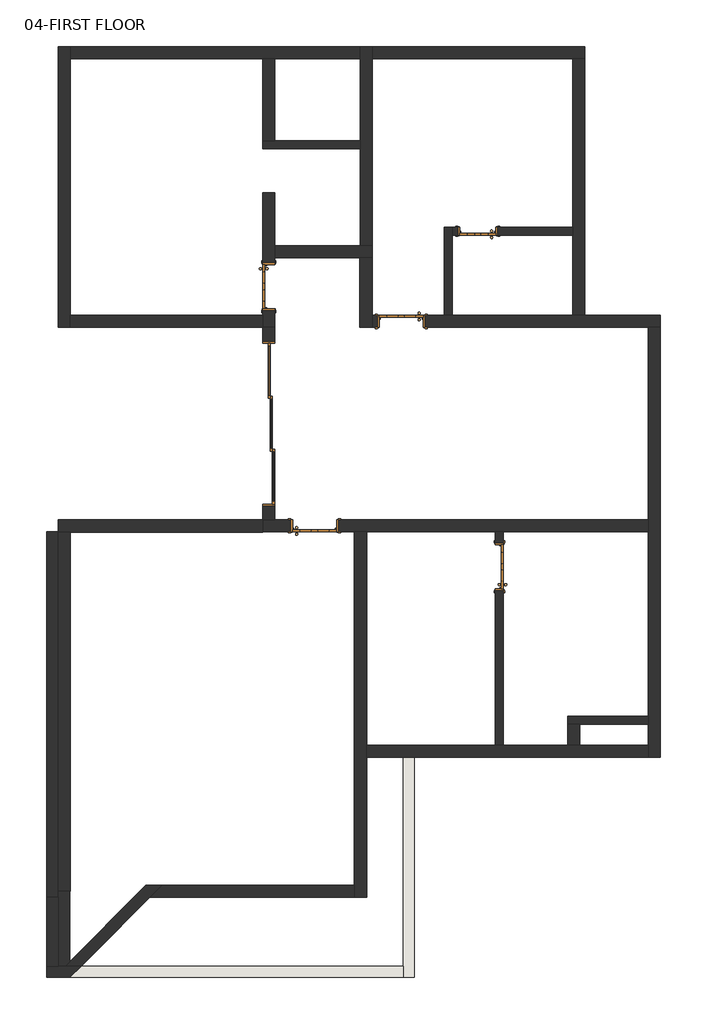
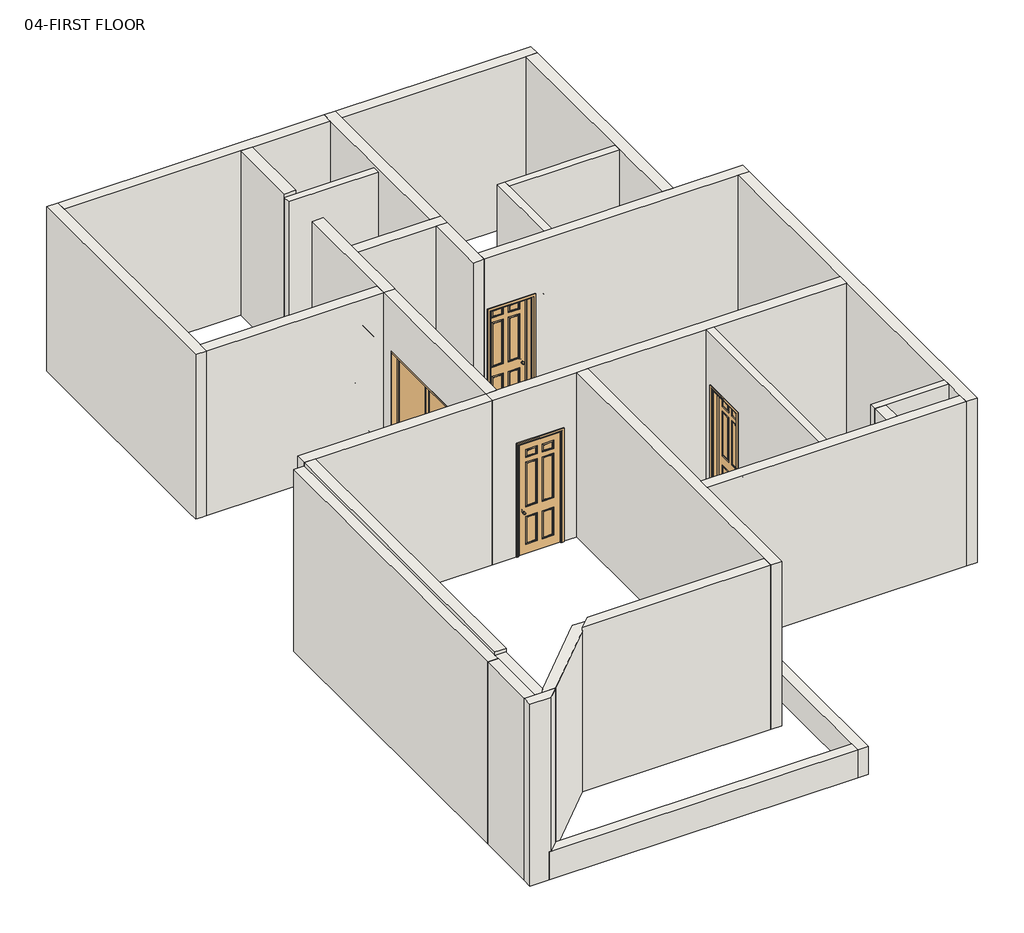
# One storey: 32 walls, 6 doors.
"""IFC4 building model written with IfcOpenShell, lengths in millimetres."""

from ifc_helpers import new_model, si_unit, frame, origin, place, context, project, spatial, polyline, outline, extrude, faceted_brep, transform, mapped, element, save
from components import d4_ba08b5a2, intsgl_9_d1_21fcec07, intsgl_9_d1_ea64c5f3, intsgl_9_d2_8283ee4d

model = new_model("IFC4")

# Units and contexts
model_context = context("Model", 3, world=origin())
ifc_project = project(units=[si_unit("LENGTHUNIT", "METRE", prefix="MILLI")], contexts=[model_context])

# Site, building, storey
site = spatial("IfcSite", under=ifc_project)
building = spatial("IfcBuilding", under=site)
storey = spatial("IfcBuildingStorey", under=building, Name="04-FIRST FLOOR", Elevation=4050.0)

# Doors
placement = place(None, origin())
d4_shape = d4_ba08b5a2(model_context)
element("IfcDoor", 1, ObjectType="D4", at=placement, inside=storey, context=model_context, shape_type="MappedRepresentation", body=[
    mapped(d4_shape, transform((-10636.6107921, -10590.6567046, 4050.0), x_axis=(0.0, 1.0, 0.0), y_axis=(-1.0, 0.0, 0.0), z_axis=(0.0, 0.0, 1.0))),
])
intsgl_9_d1_shape = intsgl_9_d1_21fcec07(model_context)
element("IfcDoor", 2, ObjectType="IntSgl (9) : D1", at=placement, inside=storey, context=model_context, shape_type="MappedRepresentation", body=[
    mapped(intsgl_9_d1_shape, transform((-8164.1107921, -8599.8987034, 4050.0), x_axis=(-1.0, 0.0, 0.0), y_axis=(0.0, -1.0, 0.0), z_axis=(0.0, 0.0, 1.0))),
])
element("IfcDoor", 3, ObjectType="IntSgl (9) : D1", at=placement, inside=storey, context=model_context, shape_type="MappedRepresentation", body=[
    mapped(intsgl_9_d1_shape, transform((-10634.1107921, -7949.8987034, 4050.0), x_axis=(0.0, -1.0, 0.0), y_axis=(1.0, 0.0, 0.0), z_axis=(0.0, 0.0, 1.0))),
])
element("IfcDoor", 4, ObjectType="IntSgl (9) : D1", at=placement, inside=storey, context=model_context, shape_type="MappedRepresentation", body=[
    mapped(intsgl_9_d1_shape, transform((-9780.3607921, -12409.8987034, 4050.0), x_axis=(1.0, 0.0, 0.0), y_axis=(0.0, 1.0, 0.0), z_axis=(0.0, 0.0, 1.0))),
])
intsgl_9_d1_2_shape = intsgl_9_d1_ea64c5f3(model_context)
element("IfcDoor", 5, ObjectType="IntSgl (9) : D1", at=placement, inside=storey, context=model_context, shape_type="MappedRepresentation", body=[
    mapped(intsgl_9_d1_2_shape, transform((-6334.1107921, -13172.3987034, 4050.0), x_axis=(0.0, 1.0, 0.0), y_axis=(-1.0, 0.0, 0.0), z_axis=(0.0, 0.0, 1.0))),
])
intsgl_9_d2_shape = intsgl_9_d2_8283ee4d(model_context)
element("IfcDoor", 6, ObjectType="IntSgl (9) : D2", at=placement, inside=storey, context=model_context, shape_type="MappedRepresentation", body=[
    mapped(intsgl_9_d2_shape, transform((-6739.1107921, -6919.8987034, 4050.0), x_axis=(-1.0, 0.0, 0.0), y_axis=(0.0, -1.0, 0.0), z_axis=(0.0, 0.0, 1.0))),
])

# Walls
element("IfcWall", 7, ObjectType="01-150 WALL", at=placement, inside=storey, context=model_context, shape_type="Brep", body=[
    faceted_brep([(-3561.6107921, -15954.8987034, 4050.0), (-5059.1107921, -15954.8987034, 4050.0), (-5059.1107921, -15954.8987034, 7575.0), (-3561.6107921, -15954.8987034, 7575.0), (-3561.6107921, -16104.8987034, 4050.0), (-3561.6107921, -16104.8987034, 7575.0), (-4834.1107921, -16104.8987034, 7575.0), (-5059.1107921, -16104.8987034, 7575.0), (-5059.1107921, -16104.8987034, 4050.0), (-4834.1107921, -16104.8987034, 4050.0)], [[[0, 1, 2, 3]], [[4, 5, 6, 7, 8, 9]], [[1, 0, 4, 9, 8]], [[3, 2, 7, 6, 5]], [[0, 3, 5, 4]], [[2, 1, 8, 7]]]),
])
element("IfcWall", 8, ObjectType="01-150 WALL", at=placement, inside=storey, context=model_context, shape_type="SweptSolid", body=[
    extrude(outline(polyline([(-16497.3987034, 7575.0), (-12522.3987034, 7575.0), (-12522.3987034, 4050.0), (-12722.3987034, 4050.0), (-12722.3987034, 6450.0), (-13622.3987034, 6450.0), (-13622.3987034, 4050.0), (-16497.3987034, 4050.0), (-16497.3987034, 7575.0)])), frame((-6409.1107921, 0.0, 0.0), z_axis=(1.0, 0.0, 0.0), x_axis=(0.0, 1.0, 0.0)), (0.0, 0.0, 1.0), 150.0),
])
element("IfcWall", 9, ObjectType="01-150 WALL", at=placement, inside=storey, context=model_context, shape_type="Brep", body=[
    faceted_brep([(-7214.1107921, -8487.3987034, 4050.0), (-7214.1107921, -6994.8987034, 4050.0), (-7214.1107921, -6844.8987034, 4050.0), (-7214.1107921, -6844.8987034, 7575.0), (-7214.1107921, -6994.8987034, 7575.0), (-7214.1107921, -8487.3987034, 7575.0), (-7364.1107921, -8487.3987034, 4050.0), (-7364.1107921, -8487.3987034, 7575.0), (-7364.1107921, -6844.8987034, 7575.0), (-7364.1107921, -6844.8987034, 4050.0)], [[[0, 1, 2, 3, 4, 5]], [[6, 7, 8, 9]], [[2, 1, 0, 6, 9]], [[5, 4, 3, 8, 7]], [[0, 5, 7, 6]], [[3, 2, 9, 8]]]),
])
element("IfcWall", 10, ObjectType="01-150 WALL", at=placement, inside=storey, context=model_context, shape_type="SweptSolid", body=[
    extrude(outline(polyline([(7575.0, -4971.6107921), (7575.0, -7214.1107921), (4050.0, -7214.1107921), (4050.0, -7114.1107921), (6150.0, -7114.1107921), (6150.0, -6364.1107921), (4050.0, -6364.1107921), (4050.0, -4971.6107921), (7575.0, -4971.6107921)])), frame((0.0, -6994.8987034, 0.0), z_axis=(0.0, 1.0, 0.0), x_axis=(0.0, 0.0, 1.0)), (0.0, 0.0, 1.0), 150.0),
])
element("IfcWall", 11, ObjectType="01-150 WALL", at=placement, inside=storey, context=model_context, shape_type="Brep", body=[
    faceted_brep([(-8931.6107921, -5229.8987034, 4050.0), (-10521.6107921, -5229.8987034, 4050.0), (-10746.6107921, -5229.8987034, 4050.0), (-10746.6107921, -5229.8987034, 7500.0), (-8931.6107921, -5229.8987034, 7500.0), (-8931.6107921, -5379.8987034, 4050.0), (-8931.6107921, -5379.8987034, 7500.0), (-10746.6107921, -5379.8987034, 7500.0), (-10746.6107921, -5379.8987034, 4050.0)], [[[0, 1, 2, 3, 4]], [[5, 6, 7, 8]], [[2, 1, 0, 5, 8]], [[4, 3, 7, 6]], [[0, 4, 6, 5]], [[3, 2, 8, 7]]]),
])
element("IfcWall", 12, ObjectType="01-225 WALL", at=placement, inside=storey, context=model_context, shape_type="Brep", body=[
    faceted_brep([(-14331.6107921, -8712.3987034, 4050.0), (-14331.6107921, -8487.3987034, 4050.0), (-14331.6107921, -3702.3987034, 4050.0), (-14331.6107921, -3477.3987034, 4050.0), (-14331.6107921, -3477.3987034, 7575.0), (-14331.6107921, -3702.3987034, 7575.0), (-14331.6107921, -8487.3987034, 7575.0), (-14331.6107921, -8712.3987034, 7575.0), (-14556.6107921, -8712.3987034, 4050.0), (-14556.6107921, -8712.3987034, 7575.0), (-14556.6107921, -3477.3987034, 7575.0), (-14556.6107921, -3477.3987034, 4050.0), (-14556.6107921, -8487.3987034, 4050.0), (-14444.1107921, -8712.3987034, 4050.0)], [[[0, 1, 2, 3, 4, 5, 6, 7]], [[8, 9, 10, 11, 12]], [[3, 2, 1, 0, 13, 8, 12, 11]], [[7, 6, 5, 4, 10, 9]], [[4, 3, 11, 10]], [[0, 7, 9, 8, 13]]]),
])
element("IfcWall", 13, ObjectType="01-225 WALL", at=placement, inside=storey, context=model_context, shape_type="Brep", body=[
    faceted_brep([(-14331.6107921, -3702.3987034, 4050.0), (-10746.6107921, -3702.3987034, 4050.0), (-10521.6107921, -3702.3987034, 4050.0), (-8931.6107921, -3702.3987034, 4050.0), (-8931.6107921, -3702.3987034, 7575.0), (-10521.6107921, -3702.3987034, 7575.0), (-10746.6107921, -3702.3987034, 7575.0), (-14331.6107921, -3702.3987034, 7575.0), (-14331.6107921, -3477.3987034, 4050.0), (-14331.6107921, -3477.3987034, 7575.0), (-8931.6107921, -3477.3987034, 7575.0), (-8931.6107921, -3477.3987034, 4050.0)], [[[0, 1, 2, 3, 4, 5, 6, 7]], [[8, 9, 10, 11]], [[3, 2, 1, 0, 8, 11]], [[7, 6, 5, 4, 10, 9]], [[0, 7, 9, 8]], [[4, 3, 11, 10]]]),
])
element("IfcWall", 14, ObjectType="01-225 WALL", at=placement, inside=storey, context=model_context, shape_type="Brep", body=[
    faceted_brep([(-10746.6107921, -3702.3987034, 4050.0), (-10746.6107921, -5229.8987034, 4050.0), (-10746.6107921, -5229.8987034, 7500.0), (-10746.6107921, -5229.8987034, 7575.0), (-10746.6107921, -3702.3987034, 7575.0), (-10521.6107921, -3702.3987034, 4050.0), (-10521.6107921, -3702.3987034, 7575.0), (-10521.6107921, -5229.8987034, 7575.0), (-10521.6107921, -5229.8987034, 4050.0)], [[[0, 1, 2, 3, 4]], [[5, 6, 7, 8]], [[1, 0, 5, 8]], [[4, 3, 7, 6]], [[0, 4, 6, 5]], [[3, 2, 1, 8, 7]]]),
])
element("IfcWall", 15, ObjectType="01-225 WALL", at=placement, inside=storey, context=model_context, shape_type="Brep", body=[
    faceted_brep([(-10746.6107921, -8487.3987034, 4050.0), (-14331.6107921, -8487.3987034, 4050.0), (-14331.6107921, -8487.3987034, 7575.0), (-10746.6107921, -8487.3987034, 7575.0), (-10746.6107921, -8712.3987034, 4050.0), (-10746.6107921, -8712.3987034, 7575.0), (-10749.1107921, -8712.3987034, 7575.0), (-14331.6107921, -8712.3987034, 7575.0), (-14331.6107921, -8712.3987034, 4050.0), (-10749.1107921, -8712.3987034, 4050.0)], [[[0, 1, 2, 3]], [[4, 5, 6, 7, 8, 9]], [[1, 0, 4, 9, 8]], [[3, 2, 7, 6, 5]], [[0, 3, 5, 4]], [[2, 1, 8, 7]]]),
])
element("IfcWall", 16, ObjectType="01-225 WALL", at=placement, inside=storey, context=model_context, shape_type="Brep", body=[
    faceted_brep([(-10521.6107921, -7412.3987034, 4050.0), (-8934.1107921, -7412.3987034, 4050.0), (-8709.1107921, -7412.3987034, 4050.0), (-8706.6107921, -7412.3987034, 4050.0), (-8706.6107921, -7412.3987034, 7575.0), (-8709.1107921, -7412.3987034, 7575.0), (-8934.1107921, -7412.3987034, 7575.0), (-10521.6107921, -7412.3987034, 7575.0), (-10521.6107921, -7187.3987034, 4050.0), (-10521.6107921, -7187.3987034, 7575.0), (-8931.6107921, -7187.3987034, 7575.0), (-8706.6107921, -7187.3987034, 7575.0), (-8706.6107921, -7187.3987034, 4050.0), (-8931.6107921, -7187.3987034, 4050.0)], [[[0, 1, 2, 3, 4, 5, 6, 7]], [[8, 9, 10, 11, 12, 13]], [[3, 2, 1, 0, 8, 13, 12]], [[7, 6, 5, 4, 11, 10, 9]], [[0, 7, 9, 8]], [[4, 3, 12, 11]]]),
])
element("IfcWall", 17, ObjectType="01-225 WALL", at=placement, inside=storey, context=model_context, shape_type="Brep", body=[
    faceted_brep([(-8931.6107921, -3477.3987034, 4050.0), (-8931.6107921, -3702.3987034, 4050.0), (-8931.6107921, -5229.8987034, 4050.0), (-8931.6107921, -5379.8987034, 4050.0), (-8931.6107921, -7187.3987034, 4050.0), (-8931.6107921, -7187.3987034, 7575.0), (-8931.6107921, -3702.3987034, 7575.0), (-8931.6107921, -3477.3987034, 7575.0), (-8706.6107921, -3477.3987034, 4050.0), (-8706.6107921, -3477.3987034, 7575.0), (-8706.6107921, -3479.8987034, 7575.0), (-8706.6107921, -3704.8987034, 7575.0), (-8706.6107921, -7187.3987034, 7575.0), (-8706.6107921, -7187.3987034, 4050.0), (-8706.6107921, -3704.8987034, 4050.0), (-8706.6107921, -3479.8987034, 4050.0)], [[[0, 1, 2, 3, 4, 5, 6, 7]], [[8, 9, 10, 11, 12, 13, 14, 15]], [[4, 3, 2, 1, 0, 8, 15, 14, 13]], [[7, 6, 5, 12, 11, 10, 9]], [[5, 4, 13, 12]], [[0, 7, 9, 8]]]),
])
element("IfcWall", 18, ObjectType="01-225 WALL", at=placement, inside=storey, context=model_context, shape_type="Brep", body=[
    faceted_brep([(-8706.6107921, -3704.8987034, 4050.0), (-4971.6107921, -3704.8987034, 4050.0), (-4746.6107921, -3704.8987034, 4050.0), (-4746.6107921, -3704.8987034, 7575.0), (-4971.6107921, -3704.8987034, 7575.0), (-8706.6107921, -3704.8987034, 7575.0), (-8706.6107921, -3479.8987034, 4050.0), (-8706.6107921, -3479.8987034, 7575.0), (-4746.6107921, -3479.8987034, 7575.0), (-4746.6107921, -3479.8987034, 4050.0)], [[[0, 1, 2, 3, 4, 5]], [[6, 7, 8, 9]], [[2, 1, 0, 6, 9]], [[5, 4, 3, 8, 7]], [[0, 5, 7, 6]], [[3, 2, 9, 8]]]),
])
element("IfcWall", 19, ObjectType="01-225 WALL", at=placement, inside=storey, context=model_context, shape_type="Brep", body=[
    faceted_brep([(-4746.6107921, -8487.3987034, 4050.0), (-4746.6107921, -3704.8987034, 4050.0), (-4746.6107921, -3704.8987034, 7575.0), (-4746.6107921, -8487.3987034, 7575.0), (-4971.6107921, -8487.3987034, 4050.0), (-4971.6107921, -8487.3987034, 7575.0), (-4971.6107921, -6994.8987034, 7575.0), (-4971.6107921, -6844.8987034, 7575.0), (-4971.6107921, -3704.8987034, 7575.0), (-4971.6107921, -3704.8987034, 4050.0), (-4971.6107921, -6844.8987034, 4050.0), (-4971.6107921, -6994.8987034, 4050.0)], [[[0, 1, 2, 3]], [[4, 5, 6, 7, 8, 9, 10, 11]], [[1, 0, 4, 11, 10, 9]], [[3, 2, 8, 7, 6, 5]], [[2, 1, 9, 8]], [[0, 3, 5, 4]]]),
])
element("IfcWall", 20, ObjectType="01-225 WALL", at=placement, inside=storey, context=model_context, shape_type="Brep", body=[
    faceted_brep([(-8934.1107921, -7412.3987034, 4050.0), (-8934.1107921, -8712.3987034, 4050.0), (-8934.1107921, -8712.3987034, 7575.0), (-8934.1107921, -7412.3987034, 7575.0), (-8709.1107921, -7412.3987034, 4050.0), (-8709.1107921, -7412.3987034, 7575.0), (-8709.1107921, -8487.3987034, 7575.0), (-8709.1107921, -8712.3987034, 7575.0), (-8709.1107921, -8712.3987034, 4050.0), (-8709.1107921, -8487.3987034, 4050.0)], [[[0, 1, 2, 3]], [[4, 5, 6, 7, 8, 9]], [[1, 0, 4, 9, 8]], [[3, 2, 7, 6, 5]], [[0, 3, 5, 4]], [[2, 1, 8, 7]]]),
])
element("IfcWall", 21, ObjectType="01-225 WALL", at=placement, inside=storey, context=model_context, shape_type="Brep", body=[
    faceted_brep([(-3336.6107921, -8712.3987034, 7575.0), (-3561.6107921, -8712.3987034, 7575.0), (-8709.1107921, -8712.3987034, 7575.0), (-8709.1107921, -8712.3987034, 4050.0), (-8614.1107921, -8712.3987034, 4050.0), (-8614.1107921, -8712.3987034, 6450.0), (-7714.1107921, -8712.3987034, 6450.0), (-7714.1107921, -8712.3987034, 4050.0), (-3561.6107921, -8712.3987034, 4050.0), (-3336.6107921, -8712.3987034, 4050.0), (-8709.1107921, -8487.3987034, 7575.0), (-7364.1107921, -8487.3987034, 7575.0), (-7214.1107921, -8487.3987034, 7575.0), (-4971.6107921, -8487.3987034, 7575.0), (-4746.6107921, -8487.3987034, 7575.0), (-3336.6107921, -8487.3987034, 7575.0), (-3336.6107921, -8487.3987034, 4050.0), (-4746.6107921, -8487.3987034, 4050.0), (-4971.6107921, -8487.3987034, 4050.0), (-7214.1107921, -8487.3987034, 4050.0), (-7364.1107921, -8487.3987034, 4050.0), (-7714.1107921, -8487.3987034, 4050.0), (-7714.1107921, -8487.3987034, 6450.0), (-8614.1107921, -8487.3987034, 6450.0), (-8614.1107921, -8487.3987034, 4050.0), (-8709.1107921, -8487.3987034, 4050.0)], [[[0, 1, 2, 3, 4, 5, 6, 7, 8, 9]], [[10, 11, 12, 13, 14, 15, 16, 17, 18, 19, 20, 21, 22, 23, 24, 25]], [[3, 25, 24, 4]], [[16, 9, 8, 7, 21, 20, 19, 18, 17]], [[2, 1, 0, 15, 14, 13, 12, 11, 10]], [[3, 2, 10, 25]], [[0, 9, 16, 15]], [[23, 5, 4, 24]], [[5, 23, 22, 6]], [[6, 22, 21, 7]]]),
])
element("IfcWall", 22, ObjectType="01-225 WALL", at=placement, inside=storey, context=model_context, shape_type="Brep", body=[
    faceted_brep([(-3561.6107921, -8712.3987034, 4050.0), (-3561.6107921, -12297.3987034, 4050.0), (-3561.6107921, -12522.3987034, 4050.0), (-3561.6107921, -15954.8987034, 4050.0), (-3561.6107921, -16104.8987034, 4050.0), (-3561.6107921, -16497.3987034, 4050.0), (-3561.6107921, -16722.3987034, 4050.0), (-3561.6107921, -16722.3987034, 7575.0), (-3561.6107921, -16497.3987034, 7575.0), (-3561.6107921, -16104.8987034, 7575.0), (-3561.6107921, -15954.8987034, 7575.0), (-3561.6107921, -12522.3987034, 7575.0), (-3561.6107921, -12297.3987034, 7575.0), (-3561.6107921, -8712.3987034, 7575.0), (-3336.6107921, -8712.3987034, 4050.0), (-3336.6107921, -8712.3987034, 7575.0), (-3336.6107921, -16722.3987034, 7575.0), (-3336.6107921, -16722.3987034, 4050.0)], [[[0, 1, 2, 3, 4, 5, 6, 7, 8, 9, 10, 11, 12, 13]], [[14, 15, 16, 17]], [[6, 5, 4, 3, 2, 1, 0, 14, 17]], [[13, 12, 11, 10, 9, 8, 7, 16, 15]], [[0, 13, 15, 14]], [[7, 6, 17, 16]]]),
])
element("IfcWall", 23, ObjectType="01-225 WALL", at=placement, inside=storey, context=model_context, shape_type="Brep", body=[
    faceted_brep([(-10749.1107921, -12297.3987034, 7575.0), (-10524.1107921, -12297.3987034, 7575.0), (-3561.6107921, -12297.3987034, 7575.0), (-3561.6107921, -12297.3987034, 4050.0), (-9330.3607921, -12297.3987034, 4050.0), (-9330.3607921, -12297.3987034, 6450.0), (-10230.3607921, -12297.3987034, 6450.0), (-10230.3607921, -12297.3987034, 4050.0), (-10524.1107921, -12297.3987034, 4050.0), (-10749.1107921, -12297.3987034, 4050.0), (-3561.6107921, -12522.3987034, 7575.0), (-6259.1107921, -12522.3987034, 7575.0), (-6409.1107921, -12522.3987034, 7575.0), (-8811.6107921, -12522.3987034, 7575.0), (-9036.6107921, -12522.3987034, 7575.0), (-10749.1107921, -12522.3987034, 7575.0), (-10749.1107921, -12522.3987034, 4050.0), (-10230.3607921, -12522.3987034, 4050.0), (-10230.3607921, -12522.3987034, 6450.0), (-9330.3607921, -12522.3987034, 6450.0), (-9330.3607921, -12522.3987034, 4050.0), (-9036.6107921, -12522.3987034, 4050.0), (-8811.6107921, -12522.3987034, 4050.0), (-6409.1107921, -12522.3987034, 4050.0), (-6259.1107921, -12522.3987034, 4050.0), (-3561.6107921, -12522.3987034, 4050.0), (-10749.1107921, -12299.8987034, 4050.0), (-10749.1107921, -12299.8987034, 7575.0)], [[[0, 1, 2, 3, 4, 5, 6, 7, 8, 9]], [[10, 11, 12, 13, 14, 15, 16, 17, 18, 19, 20, 21, 22, 23, 24, 25]], [[16, 26, 9, 8, 7, 17]], [[3, 25, 24, 23, 22, 21, 20, 4]], [[2, 1, 0, 27, 15, 14, 13, 12, 11, 10]], [[0, 9, 26, 16, 15, 27]], [[3, 2, 10, 25]], [[19, 5, 4, 20]], [[5, 19, 18, 6]], [[6, 18, 17, 7]]]),
])
element("IfcWall", 24, ObjectType="01-225 WALL", at=placement, inside=storey, context=model_context, shape_type="Brep", body=[
    faceted_brep([(-10524.1107921, -8712.3987034, 7575.0), (-10524.1107921, -12297.3987034, 7575.0), (-10524.1107921, -12297.3987034, 4050.0), (-10524.1107921, -12044.8987034, 4050.0), (-10524.1107921, -12044.8987034, 6490.0), (-10524.1107921, -8964.8987034, 6490.0), (-10524.1107921, -8964.8987034, 4050.0), (-10524.1107921, -8712.3987034, 4050.0), (-10749.1107921, -12297.3987034, 7575.0), (-10749.1107921, -8712.3987034, 7575.0), (-10749.1107921, -8712.3987034, 4050.0), (-10749.1107921, -8964.8987034, 4050.0), (-10749.1107921, -8964.8987034, 6490.0), (-10749.1107921, -12044.8987034, 6490.0), (-10749.1107921, -12044.8987034, 4050.0), (-10749.1107921, -12297.3987034, 4050.0), (-10746.6107921, -8712.3987034, 4050.0), (-10746.6107921, -8712.3987034, 7575.0)], [[[0, 1, 2, 3, 4, 5, 6, 7]], [[8, 9, 10, 11, 12, 13, 14, 15]], [[2, 15, 14, 3]], [[10, 16, 7, 6, 11]], [[1, 0, 17, 9, 8]], [[2, 1, 8, 15]], [[0, 7, 16, 10, 9, 17]], [[13, 4, 3, 14]], [[4, 13, 12, 5]], [[5, 12, 11, 6]]]),
])
element("IfcWall", 25, ObjectType="01-225 WALL", at=placement, inside=storey, context=model_context, shape_type="Brep", body=[
    faceted_brep([(-10749.1107921, -12299.8987034, 4050.0), (-14556.6107921, -12299.8987034, 4050.0), (-14556.6107921, -12299.8987034, 7575.0), (-10749.1107921, -12299.8987034, 7575.0), (-10749.1107921, -12524.8987034, 4050.0), (-10749.1107921, -12524.8987034, 7575.0), (-14331.6107921, -12524.8987034, 7575.0), (-14556.6107921, -12524.8987034, 7575.0), (-14556.6107921, -12524.8987034, 4050.0), (-14331.6107921, -12524.8987034, 4050.0), (-10749.1107921, -12522.3987034, 4050.0), (-14556.6107921, -12522.3987034, 4050.0), (-10749.1107921, -12522.3987034, 7575.0)], [[[0, 1, 2, 3]], [[4, 5, 6, 7, 8, 9]], [[1, 0, 10, 4, 9, 8, 11]], [[3, 2, 7, 6, 5, 12]], [[0, 3, 12, 5, 4, 10]], [[2, 1, 11, 8, 7]]]),
])
element("IfcWall", 26, ObjectType="01-225 WALL", at=placement, inside=storey, context=model_context, shape_type="Brep", body=[
    faceted_brep([(-9036.6107921, -12522.3987034, 4050.0), (-9036.6107921, -19107.3987034, 4050.0), (-9036.6107921, -19332.3987034, 4050.0), (-9036.6107921, -19332.3987034, 7575.0), (-9036.6107921, -19107.3987034, 7575.0), (-9036.6107921, -12522.3987034, 7575.0), (-8811.6107921, -12522.3987034, 4050.0), (-8811.6107921, -12522.3987034, 7575.0), (-8811.6107921, -16497.3987034, 7575.0), (-8811.6107921, -16722.3987034, 7575.0), (-8811.6107921, -19332.3987034, 7575.0), (-8811.6107921, -19332.3987034, 4050.0), (-8811.6107921, -16722.3987034, 4050.0), (-8811.6107921, -16497.3987034, 4050.0)], [[[0, 1, 2, 3, 4, 5]], [[6, 7, 8, 9, 10, 11, 12, 13]], [[2, 1, 0, 6, 13, 12, 11]], [[5, 4, 3, 10, 9, 8, 7]], [[0, 5, 7, 6]], [[3, 2, 11, 10]]]),
])
element("IfcWall", 27, ObjectType="01-225 WALL", at=placement, inside=storey, context=model_context, shape_type="Brep", body=[
    faceted_brep([(-9036.6107921, -19107.3987034, 4050.0), (-12624.1107921, -19107.3987034, 4050.0), (-12624.1107921, -19107.3987034, 7500.0), (-12624.1107921, -19107.3987034, 7575.0), (-9036.6107921, -19107.3987034, 7575.0), (-9036.6107921, -19332.3987034, 4050.0), (-9036.6107921, -19332.3987034, 7575.0), (-12849.1107921, -19332.3987034, 7575.0), (-12849.1107921, -19332.3987034, 4050.0)], [[[0, 1, 2, 3, 4]], [[5, 6, 7, 8]], [[1, 0, 5, 8]], [[4, 3, 7, 6]], [[0, 4, 6, 5]], [[3, 2, 1, 8, 7]]]),
])
element("IfcWall", 28, ObjectType="01-225 WALL", at=placement, inside=storey, context=model_context, shape_type="Brep", body=[
    faceted_brep([(-14331.6107921, -19219.8987034, 4050.0), (-14331.6107921, -12524.8987034, 4050.0), (-14331.6107921, -12524.8987034, 7575.0), (-14331.6107921, -19219.8987034, 7575.0), (-14556.6107921, -19219.8987034, 4050.0), (-14556.6107921, -19219.8987034, 7575.0), (-14556.6107921, -12524.8987034, 7575.0), (-14556.6107921, -12524.8987034, 4050.0), (-14341.6107921, -19219.8987034, 4050.0), (-14551.6107921, -19219.8987034, 4050.0)], [[[0, 1, 2, 3]], [[4, 5, 6, 7]], [[1, 0, 8, 9, 4, 7]], [[3, 2, 6, 5]], [[0, 3, 5, 4, 9, 8]], [[2, 1, 7, 6]]]),
])
element("IfcWall", 29, ObjectType="01-225 WALL", at=placement, inside=storey, context=model_context, shape_type="Brep", body=[
    faceted_brep([(-3561.6107921, -16497.3987034, 4050.0), (-4834.1107921, -16497.3987034, 4050.0), (-5059.1107921, -16497.3987034, 4050.0), (-6259.1107921, -16497.3987034, 4050.0), (-6409.1107921, -16497.3987034, 4050.0), (-8811.6107921, -16497.3987034, 4050.0), (-8811.6107921, -16497.3987034, 7575.0), (-6409.1107921, -16497.3987034, 7575.0), (-6259.1107921, -16497.3987034, 7575.0), (-5059.1107921, -16497.3987034, 7575.0), (-4834.1107921, -16497.3987034, 7575.0), (-3561.6107921, -16497.3987034, 7575.0), (-3561.6107921, -16722.3987034, 4050.0), (-3561.6107921, -16722.3987034, 7575.0), (-8811.6107921, -16722.3987034, 7575.0), (-8811.6107921, -16722.3987034, 4050.0)], [[[0, 1, 2, 3, 4, 5, 6, 7, 8, 9, 10, 11]], [[12, 13, 14, 15]], [[5, 4, 3, 2, 1, 0, 12, 15]], [[11, 10, 9, 8, 7, 6, 14, 13]], [[0, 11, 13, 12]], [[6, 5, 15, 14]]]),
])
element("IfcWall", 30, ObjectType="01-225 WALL", at=placement, inside=storey, context=model_context, shape_type="SweptSolid", body=[
    extrude(outline(polyline([(-4834.1107921, -16104.8987034), (-4834.1107921, -16497.3987034), (-5059.1107921, -16497.3987034), (-5059.1107921, -16104.8987034), (-4834.1107921, -16104.8987034)])), frame((0.0, 0.0, 4050.0), z_axis=(0.0, 0.0, 1.0), x_axis=(1.0, 0.0, 0.0)), (0.0, 0.0, 1.0), 3525.0),
])
element("IfcWall", 31, ObjectType="01-225 WALL", at=placement, inside=storey, context=model_context, shape_type="Brep", body=[
    faceted_brep([(-10746.6107921, -8712.3987034, 7575.0), (-10746.6107921, -8487.3987034, 7575.0), (-10746.6107921, -6199.8987034, 7575.0), (-10746.6107921, -6199.8987034, 4050.0), (-10746.6107921, -7499.8987034, 4050.0), (-10746.6107921, -7499.8987034, 6450.0), (-10746.6107921, -8399.8987034, 6450.0), (-10746.6107921, -8399.8987034, 4050.0), (-10746.6107921, -8487.3987034, 4050.0), (-10746.6107921, -8712.3987034, 4050.0), (-10521.6107921, -6199.8987034, 7575.0), (-10521.6107921, -7187.3987034, 7575.0), (-10521.6107921, -7412.3987034, 7575.0), (-10521.6107921, -8712.3987034, 7575.0), (-10521.6107921, -8712.3987034, 4050.0), (-10521.6107921, -8399.8987034, 4050.0), (-10521.6107921, -8399.8987034, 6450.0), (-10521.6107921, -7499.8987034, 6450.0), (-10521.6107921, -7499.8987034, 4050.0), (-10521.6107921, -7412.3987034, 4050.0), (-10521.6107921, -7187.3987034, 4050.0), (-10521.6107921, -6199.8987034, 4050.0), (-10524.1107921, -8712.3987034, 4050.0), (-10524.1107921, -8712.3987034, 7575.0)], [[[0, 1, 2, 3, 4, 5, 6, 7, 8, 9]], [[10, 11, 12, 13, 14, 15, 16, 17, 18, 19, 20, 21]], [[3, 21, 20, 19, 18, 4]], [[14, 22, 9, 8, 7, 15]], [[2, 1, 0, 23, 13, 12, 11, 10]], [[3, 2, 10, 21]], [[0, 9, 22, 14, 13, 23]], [[6, 16, 15, 7]], [[16, 6, 5, 17]], [[17, 5, 4, 18]]]),
])
element("IfcWall", 32, ObjectType="01-225 WALL MAIN", at=placement, inside=storey, context=model_context, shape_type="Brep", body=[
    faceted_brep([(-14766.6107921, -12522.3987034, 7500.0), (-14766.6107921, -12522.3987034, 3600.0), (-14766.6107921, -19332.3987034, 3600.0), (-14766.6107921, -19332.3987034, 7500.0), (-14556.6107921, -12522.3987034, 3600.0), (-14556.6107921, -12522.3987034, 4050.0), (-14556.6107921, -12522.3987034, 7500.0), (-14556.6107921, -19332.3987034, 7500.0), (-14556.6107921, -19332.3987034, 3600.0)], [[[0, 1, 2, 3]], [[4, 5, 6, 7, 8]], [[2, 1, 4, 8]], [[3, 2, 8, 7]], [[0, 3, 7, 6]], [[0, 6, 5, 4, 1]]]),
])
element("IfcWall", 33, ObjectType="01-225 WALL MAIN", at=placement, inside=storey, context=model_context, shape_type="SweptSolid", body=[
    extrude(outline(polyline([(-14766.6107921, -20614.8987034), (-14766.6107921, -19332.3987034), (-14556.6107921, -19332.3987034), (-14556.6107921, -20614.8987034), (-14766.6107921, -20614.8987034)])), frame((0.0, 0.0, 3600.0), z_axis=(0.0, 0.0, 1.0), x_axis=(1.0, 0.0, 0.0)), (0.0, 0.0, 1.0), 3900.0),
])
element("IfcWall", 34, ObjectType="01-225 WALL MAIN", at=placement, inside=storey, context=model_context, shape_type="Brep", body=[
    faceted_brep([(-14551.6107921, -19324.8987034, 3600.0), (-14551.6107921, -20614.8987034, 3600.0), (-14551.6107921, -20614.8987034, 7500.0), (-14551.6107921, -19219.8987034, 7500.0), (-14551.6107921, -19219.8987034, 4050.0), (-14551.6107921, -19324.8987034, 4050.0), (-14341.6107921, -19324.8987034, 3600.0), (-14341.6107921, -19324.8987034, 4050.0), (-14341.6107921, -19219.8987034, 4050.0), (-14341.6107921, -19219.8987034, 7500.0), (-14341.6107921, -20527.9138553, 7500.0), (-14341.6107921, -20527.9138553, 4050.0), (-14341.6107921, -20614.8987034, 4050.0), (-14341.6107921, -20614.8987034, 3600.0), (-14385.1032162, -20614.8987034, 3600.0), (-14428.5956402, -20614.8987034, 7500.0), (-14549.1107921, -19324.8987034, 4050.0), (-14428.5956402, -20614.8987034, 4050.0)], [[[0, 1, 2, 3, 4, 5]], [[6, 7, 8, 9, 10, 11, 12, 13]], [[1, 0, 6, 13, 14]], [[3, 2, 15, 10, 9]], [[4, 3, 9, 8]], [[4, 8, 7, 16, 5]], [[0, 5, 16, 7, 6]], [[11, 17, 12]], [[1, 14, 13, 12, 17, 15, 2]], [[15, 17, 11, 10]]]),
])
element("IfcWall", 35, ObjectType="01-225 WALL MAIN", at=placement, inside=storey, context=model_context, shape_type="Brep", body=[
    faceted_brep([(-14385.1032162, -20614.8987034, 4200.0), (-14385.1032162, -20614.8987034, 3600.0), (-14551.6107921, -20614.8987034, 3600.0), (-14556.6107921, -20614.8987034, 3600.0), (-14766.6107921, -20614.8987034, 3600.0), (-14774.1107921, -20614.8987034, 3600.0), (-14774.1107921, -20614.8987034, 7500.0), (-14766.6107921, -20614.8987034, 7500.0), (-14556.6107921, -20614.8987034, 7500.0), (-14551.6107921, -20614.8987034, 7500.0), (-14428.5956402, -20614.8987034, 7500.0), (-14131.6107921, -20614.8987034, 7500.0), (-14131.6107921, -20614.8987034, 4200.0), (-14385.1032162, -20824.8987034, 3600.0), (-14385.1032162, -20824.8987034, 4200.0), (-14341.6107921, -20824.8987034, 4200.0), (-14341.6107921, -20824.8987034, 7500.0), (-14774.1107921, -20824.8987034, 7500.0), (-14774.1107921, -20824.8987034, 3600.0)], [[[0, 1, 2, 3, 4, 5, 6, 7, 8, 9, 10, 11, 12]], [[13, 14, 15, 16, 17, 18]], [[5, 4, 3, 2, 1, 13, 18]], [[6, 5, 18, 17]], [[11, 10, 9, 8, 7, 6, 17, 16]], [[0, 14, 13, 1]], [[12, 15, 14, 0]], [[12, 11, 16, 15]]]),
])
element("IfcWall", 36, ObjectType="01-225 WALL MAIN", at=placement, inside=storey, context=model_context, shape_type="Brep", body=[
    faceted_brep([(-8129.1107921, -16722.3987034, 3600.0), (-8129.1107921, -20614.8987034, 3600.0), (-8129.1107921, -20824.8987034, 3600.0), (-8129.1107921, -20824.8987034, 4200.0), (-8129.1107921, -20614.8987034, 4200.0), (-8129.1107921, -16722.3987034, 4200.0), (-7919.1107921, -16722.3987034, 3600.0), (-7919.1107921, -16722.3987034, 4200.0), (-7919.1107921, -20824.8987034, 4200.0), (-7919.1107921, -20824.8987034, 3600.0)], [[[0, 1, 2, 3, 4, 5]], [[6, 7, 8, 9]], [[2, 1, 0, 6, 9]], [[5, 4, 3, 8, 7]], [[0, 5, 7, 6]], [[3, 2, 9, 8]]]),
])
element("IfcWall", 37, ObjectType="01-225 WALL MAIN", at=placement, inside=storey, context=model_context, shape_type="Brep", body=[
    faceted_brep([(-8129.1107921, -20614.8987034, 3600.0), (-14341.6107921, -20614.8987034, 3600.0), (-14385.1032162, -20614.8987034, 3600.0), (-14385.1032162, -20614.8987034, 4200.0), (-14131.6107921, -20614.8987034, 4200.0), (-8129.1107921, -20614.8987034, 4200.0), (-8129.1107921, -20824.8987034, 3600.0), (-8129.1107921, -20824.8987034, 4200.0), (-14341.6107921, -20824.8987034, 4200.0), (-14385.1032162, -20824.8987034, 4200.0), (-14385.1032162, -20824.8987034, 3600.0)], [[[0, 1, 2, 3, 4, 5]], [[6, 7, 8, 9, 10]], [[2, 1, 0, 6, 10]], [[5, 4, 3, 9, 8, 7]], [[0, 5, 7, 6]], [[2, 10, 9, 3]]]),
])
element("IfcWall", 38, ObjectType="01-225 WALL MAIN", at=placement, inside=storey, context=model_context, shape_type="Brep", body=[
    faceted_brep([(-14131.6107921, -20614.8987034, 7500.0), (-14131.6107921, -20614.8987034, 4200.0), (-14131.6107921, -20614.8987034, 4050.0), (-12849.1107921, -19332.3987034, 4050.0), (-12624.1107921, -19107.3987034, 4050.0), (-12624.1107921, -19107.3987034, 7500.0), (-14428.5956402, -20614.8987034, 4050.0), (-14428.5956402, -20614.8987034, 7500.0), (-14341.6107921, -20527.9138553, 7500.0), (-12921.0956402, -19107.3987034, 7500.0), (-12921.0956402, -19107.3987034, 4050.0), (-14341.6107921, -20527.9138553, 4050.0), (-14341.6107921, -20614.8987034, 4050.0)], [[[0, 1, 2, 3, 4, 5]], [[6, 7, 8, 9, 10, 11]], [[4, 3, 2, 12, 6, 11, 10]], [[0, 5, 9, 8, 7]], [[5, 4, 10, 9]], [[0, 7, 6, 12, 2, 1]]]),
])

save(model, "model.ifc")

# Revit data of these elements
# Type "D4"
#   Type Mark = "59"
#   Operation = "UserDefined"
#   Width = 3000 mm
#   Thickness = 40 mm
#   Rough Width = 3080 mm
#   Rough Height = 2440 mm
#   Panel Width = 1027.5 mm
#   Panel Frame = 55 mm
#   Height = 2400 mm
#   Frame Depth = 40 mm
#   Glass Material = Sliding Door Glass
#   Frame Material = Sliding Door Frame
#   Function = (empty or 0)
# Type "IntSgl (9) : D1"
#   Type Mark = "49"
#   Operation = "SingleSwingRight"
#   Manufacturer = "Revit"
#   Keynote = "L20"
#   UnderCut = 8 mm
#   Tolerance = 2 mm
#   Thickness = 38 mm
#   Structural Tolerance = 8 mm
#   StopDepth = 32 mm
#   Stop Thickness = 19 mm
#   Stile Top Rail = 125 mm
#   Stile Shutting = 125 mm
#   Stile Muntin Rail = 100 mm
#   Stile Lock Rail = 200 mm
#   Stile Intermediate/Frieze = 100 mm
#   Stile Hanging = 125 mm
#   Stile Bottom Rail = 200 mm
#   Rough Width = 900 mm
#   Rough Height = 2400 mm
#   Height to Top Lock Rail = 1000 mm
#   Handle Z Distance = 900 mm
#   Handle X Distance = 75 mm
#   Frame Thickness = 32 mm
#   Door Panel Width = 816 mm
#   Height = 2400 mm
#   Width = 900 mm
#   Door Panel Thickness = 38 mm
#   Door Panel Offset = 0 mm
#   Door Panel Height = 2350 mm
#   Architrave Setback = 5 mm
#   Vis - Ironmongery = yes
#   Material Ironmongery = Door - Handle
#   Material Frame = Door - Frame/Mullion
#   Material Door = Door - Panel
#   Material Architrave = Door - Architrave
#   Function = (empty or 0)
#   Wall Closure = (empty or 0)
# Type "IntSgl (9) : D2"
#   Type Mark = "50"
#   Operation = "SingleSwingRight"
#   Manufacturer = "Revit"
#   Keynote = "L20"
#   UnderCut = 8 mm
#   Tolerance = 2 mm
#   Thickness = 38 mm
#   Structural Tolerance = 8 mm
#   StopDepth = 32 mm
#   Stop Thickness = 19 mm
#   Stile Top Rail = 125 mm
#   Stile Shutting = 125 mm
#   Stile Muntin Rail = 100 mm
#   Stile Lock Rail = 200 mm
#   Stile Intermediate/Frieze = 100 mm
#   Stile Hanging = 125 mm
#   Stile Bottom Rail = 200 mm
#   Rough Width = 750 mm
#   Rough Height = 2100 mm
#   Height to Top Lock Rail = 1000 mm
#   Handle Z Distance = 900 mm
#   Handle X Distance = 75 mm
#   Frame Thickness = 32 mm
#   Door Panel Width = 666 mm
#   Height = 2100 mm
#   Width = 750 mm
#   Door Panel Thickness = 38 mm
#   Door Panel Offset = 0 mm
#   Door Panel Height = 2050 mm
#   Architrave Setback = 5 mm
#   Vis - Ironmongery = yes
#   Material Ironmongery = Door - Handle
#   Material Frame = Door - Frame/Mullion
#   Material Door = Door - Panel
#   Material Architrave = Door - Architrave
#   Function = (empty or 0)
#   Wall Closure = (empty or 0)
# Type "01-150 WALL"
#   Type Mark = "G06"
#   Layers, outside or top first: 150 mm "MY WHITE WALL PAINT" (function 1)
# Type "01-225 WALL"
#   Type Mark = "G06"
#   Layers, outside or top first: 225 mm "MY WHITE WALL PAINT" (function 1)
# Type "01-225 WALL MAIN"
#   Description = "Generic Wall (Material By Category), 200mm thick"
#   Assembly Code = "B2010"
#   Type Mark = "G06"
#   Layers, outside or top first: 5 mm "01-WHITE WALL PAINT" (function 4); 200 mm "01-DEFAULT WALL" (function 1); 5 mm "01-WHITE WALL PAINT" (function 5)
# Element 1 (IfcDoor, "D4")
#   Phase Created = New Construction
#   Materials on its faces: "Sliding Door Frame", "Sliding Door Glass"
# Elements 2, 3, 4, 5 (IfcDoor, "IntSgl (9) : D1")
#   Phase Created = New Construction
#   Materials on its faces: "Door - Panel", "Door - Architrave", "Door - Frame/Mullion", "Door - Handle"
# Element 6 (IfcDoor, "IntSgl (9) : D2")
#   Phase Created = New Construction
#   Materials on its faces: "Door - Panel", "Door - Architrave", "Door - Frame/Mullion", "Door - Handle"
# Elements 7, 8, 9, 10 (IfcWall, "01-150 WALL")
#   Top Offset = 75 mm
#   Base Offset = 0 mm
#   wall height = 3525 mm
#   Phase Created = New Construction
#   Base Constraint = 04-FIRST FLOOR
#   Materials on its faces: "MY WHITE WALL PAINT"
# Element 11 (IfcWall, "01-150 WALL")
#   Top Offset = 0 mm
#   Base Offset = 0 mm
#   wall height = 3450 mm
#   Phase Created = New Construction
#   Base Constraint = 04-FIRST FLOOR
#   Materials on its faces: "MY WHITE WALL PAINT"
# Elements 12, 13, 14, 15, 16, 17, 18, 19, 20, 21, 22, 23, 24, 25, 26, 27, 28, 29, 30, 31 (IfcWall, "01-225 WALL")
#   Top Offset = 75 mm
#   Base Offset = 0 mm
#   wall height = 3525 mm
#   Phase Created = New Construction
#   Base Constraint = 04-FIRST FLOOR
#   Materials on its faces: "MY WHITE WALL PAINT"
# Elements 32, 33, 34, 35 (IfcWall, "01-225 WALL MAIN")
#   built-in parameter 1001111 = -450 mm
#   Top Offset = 0 mm
#   Base Offset = -450 mm
#   wall height = 3900 mm
#   Phase Created = New Construction
#   Base Constraint = 04-FIRST FLOOR
#   Materials on its faces: "Default Wall", "01-WHITE WALL PAINT"
# Element 36 (IfcWall, "01-225 WALL MAIN")
#   built-in parameter 1001111 = -450 mm
#   Top Offset = 150 mm
#   Base Offset = -450 mm
#   wall height = 600 mm
#   Phase Created = New Construction
#   Base Constraint = 04-FIRST FLOOR
#   Top Constraint = 04-FIRST FLOOR
#   Materials on its faces: "01-WHITE WALL PAINT", "Default Wall"
# Element 37 (IfcWall, "01-225 WALL MAIN")
#   built-in parameter 1001111 = -450 mm
#   Top Offset = 150 mm
#   Base Offset = -450 mm
#   wall height = 600 mm
#   Phase Created = New Construction
#   Base Constraint = 04-FIRST FLOOR
#   Top Constraint = 04-FIRST FLOOR
#   Materials on its faces: "Default Wall", "01-WHITE WALL PAINT"
# Element 38 (IfcWall, "01-225 WALL MAIN")
#   Top Offset = 0 mm
#   Base Offset = 0 mm
#   wall height = 3450 mm
#   Phase Created = New Construction
#   Base Constraint = 04-FIRST FLOOR
#   Materials on its faces: "Default Wall", "01-WHITE WALL PAINT", "MY WHITE WALL PAINT"
# Materials
#   "Sliding Door Glass": colour RGB 247 247 247, transparency 0.68
#   "Sliding Door Frame": colour RGB 160 107 8, transparency 0
#   "Door - Handle": colour RGB 0 0 0, transparency 0, Keynote = "P21", Cost = 0, Export to IFC = 0
#   "Door - Frame/Mullion": class "Wood", colour RGB 212 179 113, transparency 0, Keynote = "L20", Cost = 0, Export to IFC = 0
#   "Door - Panel": class "Wood", colour RGB 210 159 95, transparency 0, Keynote = "L20", Cost = 0, Export to IFC = 0
#   "Door - Architrave": class "Wood", colour RGB 154 90 5, transparency 0, Keynote = "P20", Cost = 0, Export to IFC = 0
#   "MY WHITE WALL PAINT": class "Gas", colour RGB 0 0 0, transparency 0, Description = "Air", Cost = 0
#   "01-WHITE WALL PAINT": class "Generic", colour RGB 0 0 0, transparency 0, Description = "Acoustic Ceiling Tile 24 x 48", Cost = 0
#   "01-DEFAULT WALL": class "Generic", colour RGB 242 242 255, transparency 0, Description = "Acoustic Ceiling Tile 24 x 48", Cost = 0
#   "Default Wall": colour RGB 128 128 128, transparency 0, Cost = 0, Export to IFC = 0
